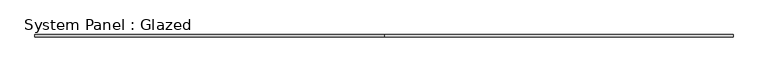
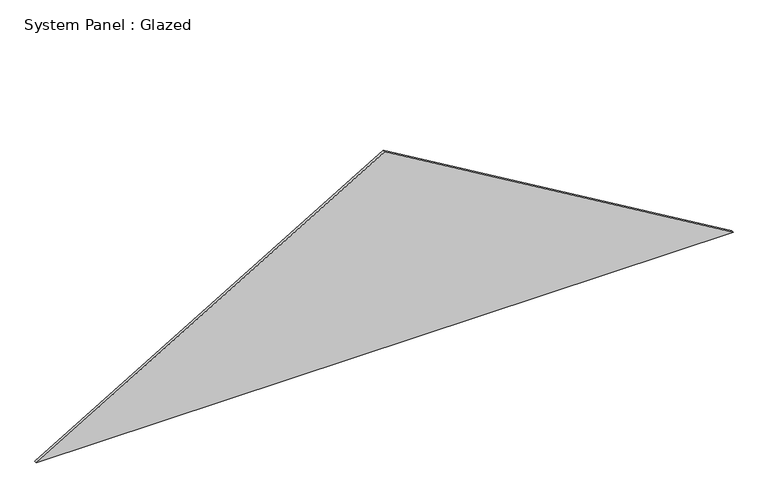
"""IFC4 building model written with IfcOpenShell, lengths in millimetres: plate geometry, System Panel : Glazed."""

from ifc_helpers import new_model, si_unit, frame, origin, place, context, project, spatial, polyline, outline, extrude, source, transform, mapped, element, save


def system_panel_glazed_4284b2b2(model_context):
    return source(origin(), model_context, "Body", "SweptSolid", [
        extrude(outline(polyline([(0.0, -3580.0175257), (0.0, 3580.0175257), (2127.7626397, 0.0), (0.0, -3580.0175257)])), frame((0.0, 19.05, 0.0), z_axis=(0.0, 1.0, 0.0), x_axis=(0.0, 0.0, 1.0)), (0.0, 0.0, 1.0), 25.4),
    ])


if __name__ == "__main__":
    model = new_model("IFC4")
    model_context = context("Model", 3, world=origin())
    ifc_project = project(units=[si_unit("LENGTHUNIT", "METRE", prefix="MILLI")], contexts=[model_context])
    site = spatial("IfcSite", under=ifc_project)
    building = spatial("IfcBuilding", under=site)
    placement = place(None, origin())
    system_panel_glazed_shape = system_panel_glazed_4284b2b2(model_context)
    element("IfcPlate", 1, ObjectType="System Panel : Glazed", at=placement, inside=building, context=model_context, shape_type="MappedRepresentation", body=[
        mapped(system_panel_glazed_shape, transform((0.0, 0.0, 0.0), x_axis=(1.0, 0.0, 0.0), y_axis=(0.0, 1.0, 0.0), z_axis=(0.0, 0.0, 1.0))),
    ])
    save(model, "model.ifc")

# Revit data of these elements
# Type "System Panel : Glazed"
#   Construction Type Id = "GSP4R"
#   Analytic Construction = "1/8 in Pilkington single glazing"
#   Visual Light Transmittance = 0.9
#   Solar Heat Gain Coefficient = 0.86
#   Heat Transfer Coefficient (U) = 1.18115 BTU/(h·ft²·°F)
#   Define Thermal Properties by = 1
# Element 1 (IfcPlate, "System Panel : Glazed")
#   Materials on its faces: "Glass"
# Materials
#   "Glass": class "Glass", colour RGB 0 128 192, transparency 0.75, Description = "Soda Lime Glass", Cost = 0
